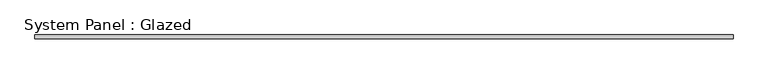
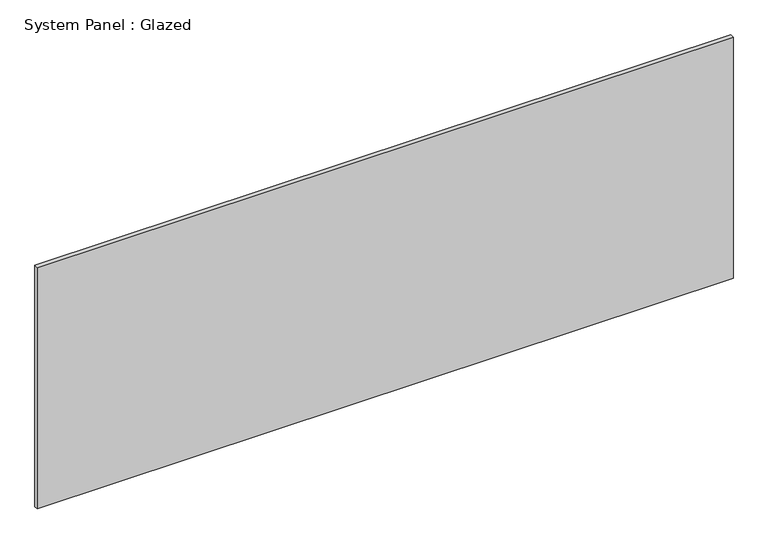
"""IFC4 building model written with IfcOpenShell, lengths in millimetres: plate geometry, System Panel : Glazed."""

from ifc_helpers import new_model, si_unit, origin, origin_with_axes, place, context, project, spatial, polyline, outline, extrude, source, transform, mapped, element, save


def system_panel_glazed_5a8eca4b(model_context):
    return source(origin(), model_context, "Body", "SweptSolid", [
        extrude(outline(polyline([(2406.65, 19.05), (-2406.65, 19.05), (-2406.65, 44.45), (2406.65, 44.45), (2406.65, 19.05)])), origin_with_axes(), (0.0, 0.0, 1.0), 1765.3),
    ])


if __name__ == "__main__":
    model = new_model("IFC4")
    model_context = context("Model", 3, world=origin())
    ifc_project = project(units=[si_unit("LENGTHUNIT", "METRE", prefix="MILLI")], contexts=[model_context])
    site = spatial("IfcSite", under=ifc_project)
    building = spatial("IfcBuilding", under=site)
    placement = place(None, origin())
    system_panel_glazed_shape = system_panel_glazed_5a8eca4b(model_context)
    element("IfcPlate", 1, ObjectType="System Panel : Glazed", at=placement, inside=building, context=model_context, shape_type="MappedRepresentation", body=[
        mapped(system_panel_glazed_shape, transform((0.0, 0.0, 0.0), x_axis=(1.0, 0.0, 0.0), y_axis=(0.0, 1.0, 0.0), z_axis=(0.0, 0.0, 1.0))),
    ])
    save(model, "model.ifc")

# Revit data of these elements
# Type "System Panel : Glazed"
#   Construction Type Id = "GSP4R"
#   Analytic Construction = "1/8 in Pilkington single glazing"
#   Visual Light Transmittance = 0.9
#   Solar Heat Gain Coefficient = 0.86
#   Heat Transfer Coefficient (U) = 1.18115 BTU/(h·ft²·°F)
# Element 1 (IfcPlate, "System Panel : Glazed")
#   Materials on its faces: "Glass"
# Materials
#   "Glass": class "Glass", colour RGB 0 128 192, transparency 0.75, Description = "Soda Lime Glass", Cost = 0
